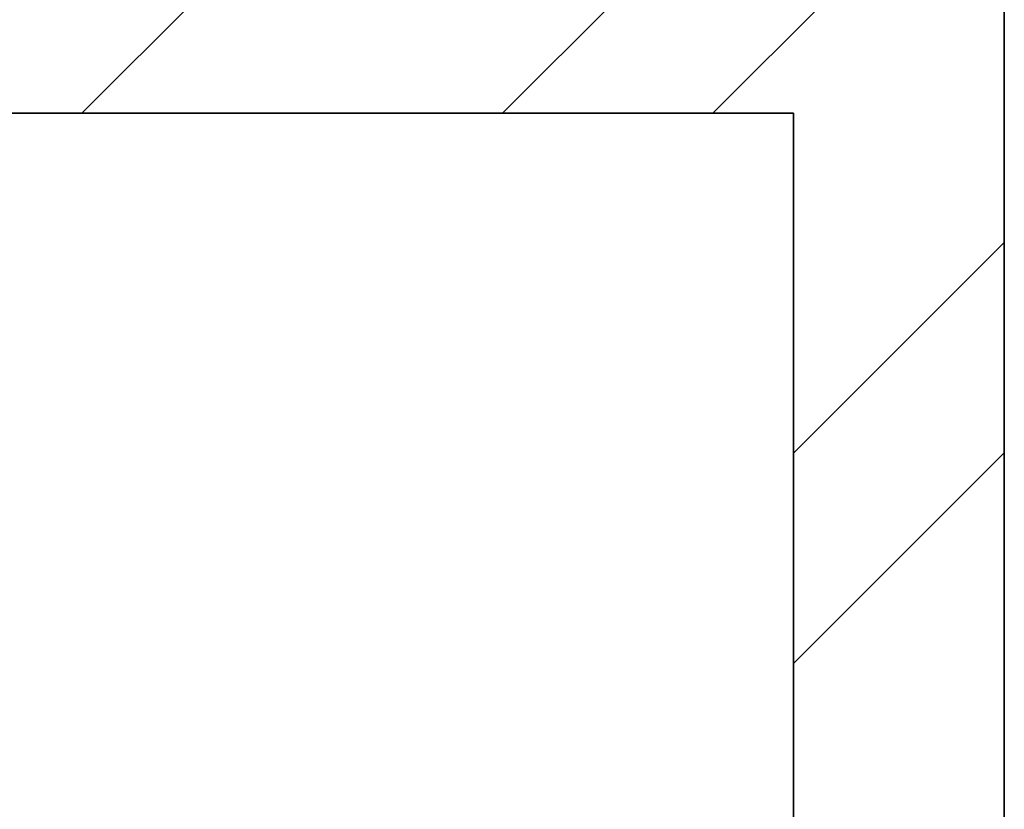
# Model space of a CAD drawing. Units: inches. Extents: x 2168 to 3056, y 1130 to 2629.
# Tile 38 of 42: x 2843 to 2864, y 2246 to 2263. Entities that reach past the tile are written whole.
import ezdxf

# ---------------------------------------------------------------- set-up
doc = ezdxf.new("R2010")
doc.units = ezdxf.units.IN
doc.layers.add('A-WALL', color=7, linetype='Continuous', lineweight=35)
doc.layers.add('A-WALL-PATT', color=143, linetype='Continuous', lineweight=13, true_color=0x7aafdf)

msp = doc.modelspace()

# ---------------------------------------------------------------- hatches: boundary and pattern name
at = {"layer": 'A-WALL-PATT'}
h = msp.add_hatch(dxfattribs=at)
h.set_pattern_fill('ANSI32', color=256)
h.paths.add_polyline_path([(2463.796, 2409.389), (2467.387, 2409.389), (2467.387, 2413.889), (2454.768, 2413.889), (2454.768, 2411.639), (2454.768, 2409.389), (2459.296, 2409.389), (2459.296, 2265.389), (2455.644, 2265.389), (2455.644, 2260.889), (2467.349, 2260.889), (2467.349, 2263.139), (2467.349, 2265.389), (2463.796, 2265.389)])
h.paths.add_polyline_path([(2431.596, 2413.889), (2409.647, 2413.889), (2409.647, 2409.389), (2431.596, 2409.389), (2431.596, 2411.639)])
h.paths.add_polyline_path([(2349.647, 2413.889), (2331.796, 2413.889), (2331.796, 2362.671), (2336.296, 2362.671), (2336.296, 2409.389), (2349.647, 2409.389), (2349.647, 2411.639)])
h.paths.add_polyline_path([(2634.149, 2411.639), (2634.149, 2413.889), (2562.293, 2413.889), (2562.293, 2409.389), (2595.796, 2409.389), (2595.796, 2280.309), (2595.826, 2280.309), (2595.826, 2265.389), (2499.91, 2265.389), (2499.91, 2260.889), (2550.796, 2260.889), (2550.796, 2117.308), (2555.296, 2117.308), (2555.296, 2168.08), (2571.93, 2168.08), (2571.93, 2176.889), (2559.796, 2176.889), (2559.796, 2256.389), (2640.796, 2256.389), (2640.796, 2176.889), (2626.428, 2176.889), (2626.428, 2168.08), (2645.296, 2168.08), (2645.296, 2116.637), (2649.796, 2116.637), (2649.796, 2260.889), (2691.251, 2260.889), (2691.251, 2263.139), (2691.251, 2265.389), (2670.655, 2265.389), (2670.655, 2265.365), (2600.296, 2265.365), (2600.296, 2280.258), (2600.296, 2409.389), (2634.149, 2409.389)])
h.paths.add_polyline_path([(2600.296, 2473.889), (2612.84, 2473.889), (2612.84, 2478.389), (2572.636, 2478.389), (2572.636, 2473.889), (2595.796, 2473.889), (2595.796, 2413.889), (2600.296, 2413.889)])
h.paths.add_polyline_path([(2535.796, 2473.889), (2548.636, 2473.889), (2548.636, 2478.389), (2531.396, 2478.389), (2531.396, 2413.889), (2521.6, 2413.889), (2521.6, 2409.389), (2539.239, 2409.389), (2539.239, 2411.639), (2539.239, 2413.889), (2535.796, 2413.889)])
h.paths.add_polyline_path([(2664.796, 2478.389), (2636.84, 2478.389), (2636.84, 2473.889), (2660.296, 2473.889), (2660.296, 2413.889), (2656.165, 2413.889), (2656.165, 2409.389), (2671.684, 2409.389), (2671.684, 2411.639), (2671.684, 2413.889), (2664.796, 2413.889)])
h.paths.add_polyline_path([(2705.942, 2413.889), (2695.684, 2413.889), (2695.684, 2409.389), (2705.942, 2409.389)])
h.paths.add_polyline_path([(2741.35, 2413.889), (2728.733, 2413.889), (2728.733, 2411.639), (2728.733, 2409.389), (2732.296, 2409.389), (2732.296, 2265.389), (2725.733, 2265.389), (2725.733, 2260.889), (2740.917, 2260.889), (2740.917, 2263.139), (2740.917, 2265.389), (2736.796, 2265.389), (2736.796, 2409.389), (2741.35, 2409.389)])
h.paths.add_polyline_path([(2785.655, 2413.889), (2764.546, 2413.889), (2764.486, 2409.389), (2785.655, 2409.389), (2785.655, 2411.639)])
h.paths.add_polyline_path([(2864.296, 2413.889), (2845.655, 2413.889), (2845.655, 2409.389), (2859.796, 2409.389), (2859.796, 2368.425), (2864.296, 2368.425)])
h.paths.add_polyline_path([(2864.296, 2308.425), (2862.046, 2308.425), (2859.796, 2308.425), (2859.796, 2265.389), (2774.483, 2265.389), (2774.483, 2263.139), (2774.483, 2260.889), (2781.796, 2260.889), (2781.796, 2226.654), (2786.296, 2226.654), (2786.296, 2260.889), (2859.796, 2260.889), (2859.796, 2241.352), (2864.296, 2241.352)])
h.paths.add_polyline_path([(2864.296, 2217.352), (2862.046, 2217.352), (2859.796, 2217.352), (2859.796, 2200.889), (2786.296, 2200.889), (2786.296, 2205.931), (2784.046, 2205.931), (2781.796, 2205.931), (2781.796, 2150.974), (2786.296, 2150.974), (2786.296, 2161.889), (2859.796, 2161.889), (2859.796, 2144.419), (2864.296, 2144.419)])
h.paths.add_polyline_path([(2859.796, 2196.389), (2859.796, 2166.389), (2786.296, 2166.389), (2786.296, 2196.389)], flags=16)
h.paths.add_polyline_path([(2864.296, 2108.419), (2862.046, 2108.419), (2859.796, 2108.419), (2859.796, 2080.889), (2786.296, 2080.889), (2786.296, 2111.993), (2781.796, 2111.993), (2781.796, 2080.889), (2649.796, 2080.889), (2649.796, 2086.036), (2647.546, 2086.036), (2645.296, 2086.036), (2645.296, 2071.739), (2649.796, 2071.739), (2649.796, 2076.389), (2781.796, 2076.389), (2781.796, 2041.792), (2786.296, 2041.792), (2786.296, 2076.389), (2859.796, 2076.389), (2859.796, 2058.577), (2864.296, 2058.577)])
h.paths.add_polyline_path([(2864.296, 2022.577), (2859.796, 2022.577), (2859.796, 1992.389), (2786.296, 1992.389), (2786.296, 1999.573), (2781.796, 1999.573), (2781.796, 1848.085), (2784.046, 1848.085), (2786.296, 1848.085), (2786.296, 1851.389), (2859.796, 1851.389), (2859.796, 1838.258), (2864.296, 1838.258)], flags=17)
h.paths.add_polyline_path([(2859.796, 1987.889), (2859.796, 1855.889), (2786.296, 1855.889), (2786.296, 1987.889)], flags=16)
h.paths.add_polyline_path([(2823.046, 1987.889), (2841.421, 1921.889), (2823.046, 1855.889)], flags=0)
h.paths.add_polyline_path([(2864.296, 1814.258), (2859.796, 1814.258), (2859.796, 1791.389), (2786.296, 1791.389), (2786.296, 1825.658), (2784.046, 1825.658), (2781.796, 1825.658), (2781.796, 1791.389), (2720.155, 1791.389), (2720.155, 1791.265), (2649.796, 1791.265), (2649.796, 1806.159), (2649.796, 2038.983), (2647.546, 2038.983), (2645.296, 2038.983), (2645.296, 1783.925), (2649.796, 1783.925), (2649.796, 1786.889), (2781.796, 1786.889), (2781.796, 1746.789), (2786.296, 1746.789), (2786.296, 1786.889), (2859.796, 1786.889), (2859.796, 1770.083), (2864.296, 1770.083)])
h.paths.add_polyline_path([(2864.296, 1734.083), (2862.046, 1734.083), (2859.796, 1734.083), (2859.796, 1705.889), (2786.296, 1705.889), (2786.296, 1714.166), (2781.796, 1714.166), (2781.796, 1660.527), (2786.296, 1660.527), (2786.296, 1666.889), (2859.796, 1666.889), (2859.796, 1648.342), (2864.296, 1648.342)])
h.paths.add_polyline_path([(2786.296, 1701.389), (2859.796, 1701.389), (2859.796, 1671.389), (2786.296, 1671.389)], flags=16)
h.paths.add_polyline_path([(2649.796, 1756.576), (2647.546, 1756.576), (2645.296, 1756.576), (2645.296, 1606.889), (2555.296, 1606.889), (2555.296, 1749.513), (2553.046, 1749.513), (2550.796, 1749.513), (2550.796, 1606.889), (2503.006, 1606.889), (2503.006, 1604.639), (2503.006, 1602.389), (2595.796, 1602.389), (2595.849, 1602.389), (2595.849, 1587.495), (2595.796, 1458.389), (2561.502, 1458.389), (2561.502, 1456.139), (2561.502, 1453.889), (2595.796, 1453.889), (2595.796, 1381.889), (2573.438, 1381.889), (2573.438, 1377.389), (2613.01, 1377.389), (2613.01, 1379.639), (2613.01, 1381.889), (2600.296, 1381.889), (2600.296, 1453.889), (2634.327, 1453.889), (2634.327, 1458.389), (2600.296, 1458.389), (2600.296, 1602.389), (2670.655, 1602.389), (2694.095, 1602.389), (2694.095, 1606.889), (2649.796, 1606.889)])
h.paths.add_polyline_path([(2736.796, 1602.389), (2741.562, 1602.389), (2741.562, 1606.889), (2726.203, 1606.889), (2726.203, 1604.639), (2726.203, 1602.389), (2732.296, 1602.389), (2732.296, 1458.389), (2727.899, 1458.389), (2727.899, 1453.889), (2740.821, 1453.889), (2740.821, 1456.139), (2740.821, 1458.389), (2736.796, 1458.389)])
h.paths.add_polyline_path([(2859.796, 1606.889), (2786.296, 1606.889), (2786.296, 1637.334), (2784.046, 1637.334), (2781.796, 1637.334), (2781.796, 1606.889), (2775.612, 1606.889), (2775.612, 1602.389), (2859.796, 1602.389)])
h.paths.add_polyline_path([(2864.296, 1624.342), (2862.046, 1624.342), (2859.796, 1624.342), (2859.796, 1570.39), (2864.296, 1570.39)])
h.paths.add_polyline_path([(2864.296, 1510.39), (2862.046, 1510.39), (2859.796, 1510.39), (2859.796, 1458.389), (2846.735, 1458.389), (2846.735, 1456.139), (2846.735, 1453.889), (2864.296, 1453.889)])
h.paths.add_polyline_path([(2786.735, 1458.389), (2765.444, 1458.389), (2765.444, 1453.889), (2786.735, 1453.889)])
h.paths.add_polyline_path([(2706.004, 1458.389), (2695.36, 1458.389), (2695.36, 1453.889), (2706.004, 1453.889), (2706.004, 1456.139)])
h.paths.add_polyline_path([(2671.36, 1456.139), (2671.36, 1458.389), (2655.986, 1458.389), (2655.986, 1456.139), (2655.986, 1453.889), (2660.296, 1453.889), (2660.296, 1381.889), (2637.01, 1381.889), (2637.01, 1377.389), (2664.796, 1377.389), (2664.796, 1453.889), (2671.36, 1453.889)], flags=17)
h.paths.add_polyline_path([(2539.829, 1458.389), (2520.237, 1458.389), (2520.237, 1453.889), (2531.296, 1453.889), (2531.296, 1377.389), (2546.449, 1377.389), (2546.449, 1379.639), (2546.449, 1381.889), (2535.796, 1381.889), (2535.796, 1453.889), (2539.829, 1453.889)], flags=17)
h.paths.add_polyline_path([(2496.237, 1458.389), (2489.13, 1458.389), (2489.13, 1453.889), (2496.237, 1453.889), (2496.237, 1456.139)])
h.paths.add_polyline_path([(2467.433, 1456.139), (2467.433, 1458.389), (2463.796, 1458.389), (2463.796, 1602.389), (2468.242, 1602.389), (2468.242, 1605.7), (2468.242, 1606.889), (2454.602, 1606.889), (2454.602, 1602.389), (2459.296, 1602.389), (2459.296, 1458.389), (2454.24, 1458.389), (2454.24, 1453.889), (2467.433, 1453.889)])
h.paths.add_polyline_path([(2431.601, 1456.139), (2431.601, 1458.389), (2411.386, 1458.389), (2411.386, 1453.889), (2431.601, 1453.889)])
h.paths.add_polyline_path([(2351.386, 1458.389), (2336.296, 1458.389), (2336.296, 1490.693), (2334.046, 1490.693), (2331.796, 1490.693), (2331.796, 1453.889), (2351.386, 1453.889), (2351.386, 1456.139)])
h.paths.add_polyline_path([(2336.296, 1629.705), (2331.796, 1629.705), (2331.796, 1552.317), (2336.296, 1552.317), (2336.296, 1602.389), (2406.655, 1602.389), (2423.472, 1602.389), (2423.472, 1606.889), (2418.796, 1606.889), (2418.796, 1643.678), (2416.546, 1643.678), (2414.296, 1643.678), (2414.296, 1606.889), (2336.296, 1606.889)])
h.paths.add_polyline_path([(2418.796, 1714.384), (2414.296, 1714.384), (2414.296, 1705.889), (2336.296, 1705.889), (2336.296, 1731.324), (2334.046, 1731.324), (2331.796, 1731.324), (2331.796, 1653.705), (2334.046, 1653.705), (2336.296, 1653.705), (2336.296, 1666.889), (2414.296, 1666.889), (2414.296, 1663.589), (2418.796, 1663.589)])
h.paths.add_polyline_path([(2336.296, 1701.389), (2414.296, 1701.389), (2414.296, 1671.389), (2336.296, 1671.389)], flags=16)
h.paths.add_polyline_path([(2555.296, 2040.059), (2550.796, 2040.059), (2550.796, 1791.389), (2550.561, 1791.205), (2480.202, 1791.205), (2418.796, 1791.389), (2418.796, 1825.448), (2416.546, 1825.448), (2414.296, 1825.448), (2414.296, 1791.389), (2336.296, 1791.389), (2336.296, 1806.409), (2331.796, 1806.409), (2331.796, 1767.324), (2336.296, 1767.324), (2336.296, 1786.889), (2414.296, 1786.889), (2414.296, 1745.457), (2418.796, 1745.457), (2418.796, 1786.889), (2550.796, 1786.889), (2550.796, 1783.011), (2555.296, 1783.011)])
h.paths.add_polyline_path([(2418.796, 1923.389), (2423.207, 1923.389), (2423.207, 1925.639), (2423.207, 1927.889), (2418.796, 1927.889), (2418.796, 2000.048), (2414.296, 2000.048), (2414.296, 1992.389), (2336.296, 1992.389), (2336.296, 1987.889), (2414.296, 1987.889), (2414.296, 1855.889), (2336.296, 1855.889), (2336.296, 1851.389), (2414.296, 1851.389), (2414.296, 1846.759), (2418.796, 1846.759)], flags=17)
h.paths.add_polyline_path([(2336.296, 2019.294), (2334.046, 2019.294), (2331.796, 2019.294), (2331.796, 1830.409), (2336.296, 1830.409)], flags=17)
h.paths.add_polyline_path([(2550.796, 1927.889), (2453.541, 1927.889), (2453.541, 1925.639), (2453.541, 1923.389), (2550.796, 1923.389)], flags=17)
h.paths.add_polyline_path([(2744.987, 1927.889), (2649.796, 1927.889), (2649.796, 1923.389), (2744.987, 1923.389), (2744.987, 1925.639)], flags=17)
h.paths.add_polyline_path([(2555.296, 2086.458), (2553.046, 2086.458), (2550.796, 2086.458), (2550.796, 2080.889), (2418.796, 2080.889), (2336.296, 2080.889), (2336.296, 2115.399), (2334.046, 2115.399), (2331.796, 2115.399), (2331.796, 2055.294), (2336.296, 2055.294), (2336.296, 2076.389), (2550.796, 2076.389), (2550.796, 2071.538), (2555.296, 2071.538)])
h.paths.add_polyline_path([(2418.796, 2121.389), (2414.296, 2121.389), (2414.296, 2080.889), (2418.796, 2080.889)])
h.paths.add_polyline_path([(2418.796, 2076.389), (2414.296, 2076.389), (2414.296, 2035.123), (2418.796, 2035.123)])
h.paths.add_polyline_path([(2422.868, 2263.139), (2422.868, 2265.389), (2406.655, 2265.389), (2406.655, 2265.359), (2336.296, 2265.359), (2336.296, 2280.252), (2336.296, 2302.671), (2334.046, 2302.671), (2331.796, 2302.671), (2331.796, 2246.853), (2336.296, 2246.853), (2336.296, 2260.889), (2414.296, 2260.889), (2414.296, 2223.996), (2418.796, 2223.996), (2418.796, 2260.889), (2422.868, 2260.889)])
h.paths.add_polyline_path([(2418.796, 2204.783), (2416.546, 2204.783), (2414.296, 2204.783), (2414.296, 2200.889), (2336.296, 2200.889), (2336.296, 2220.853), (2331.796, 2220.853), (2331.796, 2151.399), (2336.296, 2151.399), (2336.296, 2161.889), (2414.296, 2161.889), (2414.296, 2153.726), (2418.796, 2153.726)])
h.paths.add_polyline_path([(2414.296, 2196.389), (2414.296, 2166.389), (2336.296, 2166.389), (2336.296, 2196.389)], flags=16)
h.paths.add_polyline_path([(2375.296, 2181.389), (2336.296, 2166.389), (2336.296, 2196.389)], flags=0)
h.paths.add_polyline_path([(2809.595, 2172.34), (2838.804, 2172.34), (2838.804, 2190.997), (2809.595, 2190.997)], flags=8)
h.paths.add_polyline_path([(2849.75, 1919.585), (2849.75, 1952.672), (2831.093, 1952.672), (2831.093, 1919.585)], flags=8)
h.paths.add_polyline_path([(2808.875, 1901.967), (2808.875, 1937.85), (2790.149, 1937.85), (2790.149, 1901.967)], flags=8)
h.paths.add_polyline_path([(2806.285, 1671.896), (2835.493, 1671.896), (2835.493, 1690.553), (2806.285, 1690.553)], flags=8)
h.paths.add_polyline_path([(2353.186, 1676.549), (2382.395, 1676.549), (2382.395, 1695.207), (2353.186, 1695.207)], flags=8)
h.paths.add_polyline_path([(2360.083, 1832.308), (2389.241, 1832.308), (2389.241, 1850.966), (2360.083, 1850.966)], flags=25)
h.paths.add_polyline_path([(2354.822, 2167.823), (2384.031, 2167.823), (2384.031, 2186.481), (2354.822, 2186.481)], flags=8)

# ---------------------------------------------------------------- linework, layer by layer
at = {"layer": 'A-WALL'}
for p, q in [((2864.296, 2308.425), (2864.296, 2241.352)), ((2786.296, 2260.889), (2859.796, 2260.889)), ((2859.796, 2260.889), (2859.796, 2241.352))]:
    msp.add_line(p, q, dxfattribs=at)

doc.saveas('drawing.dxf')
